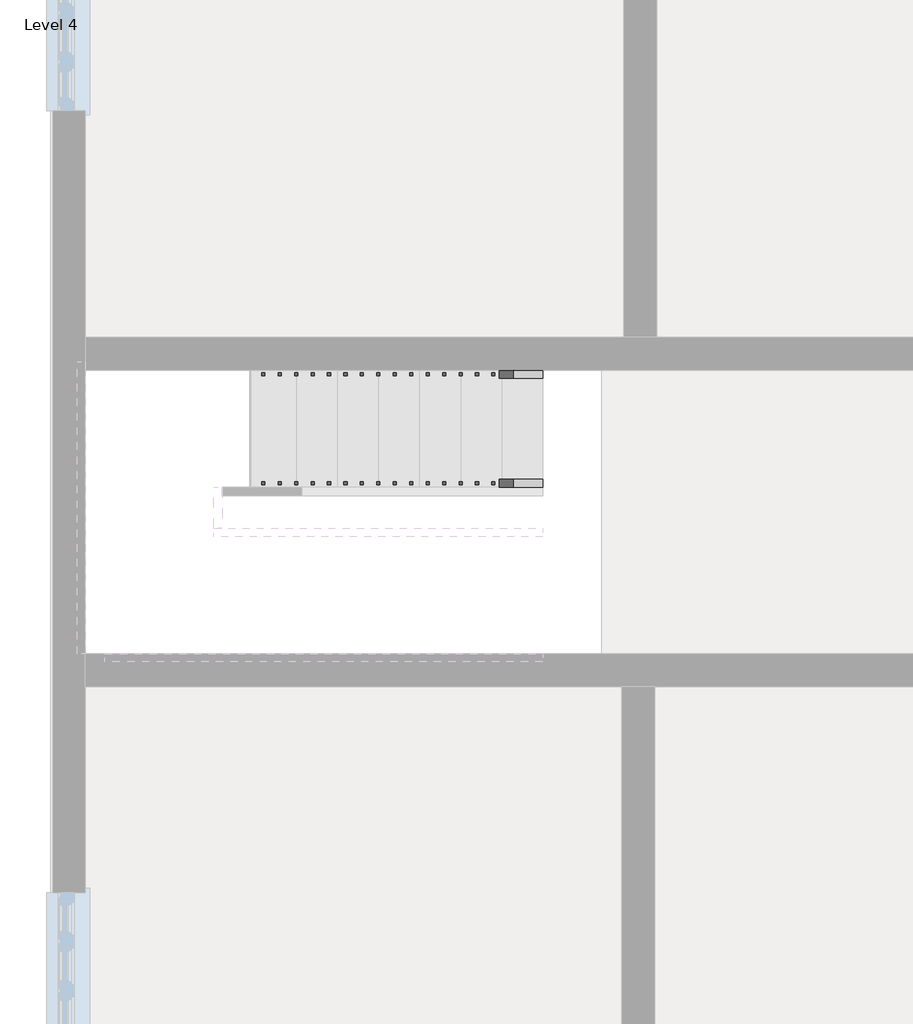
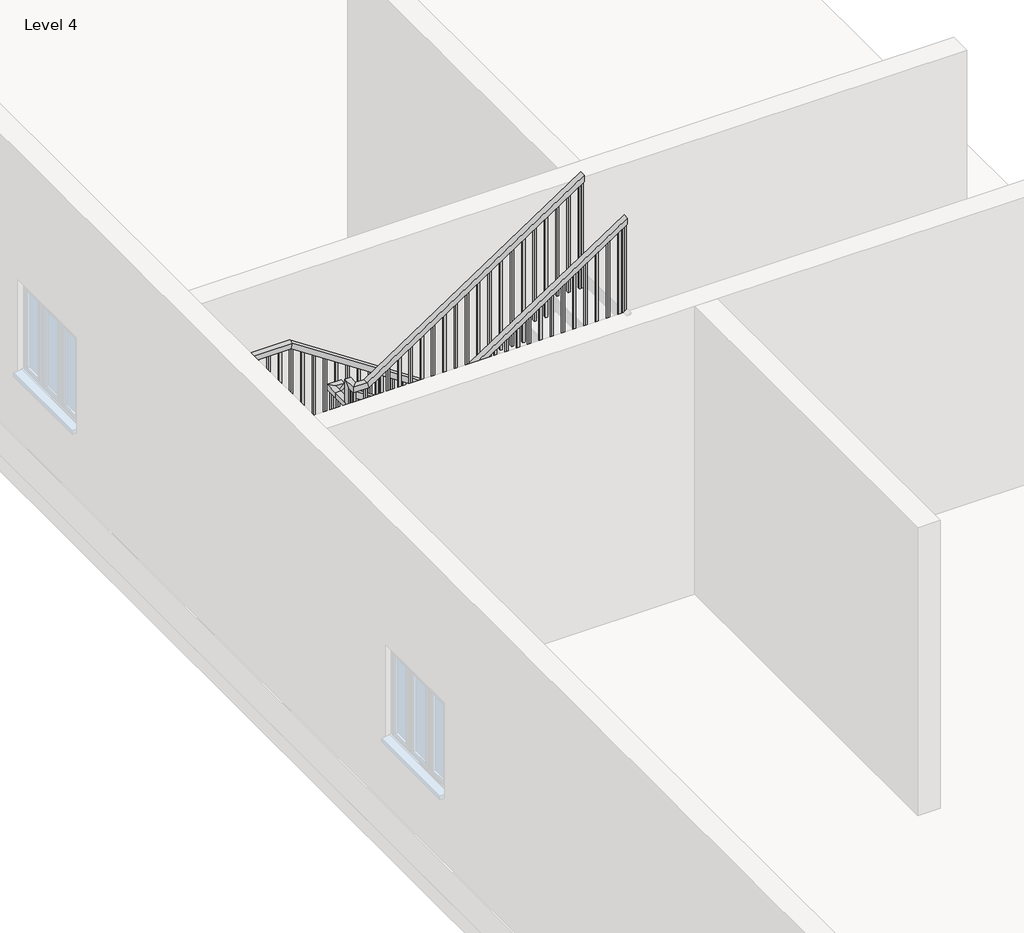
# One storey, part 2 of 3: 2 railings.
"""IFC4 building model written with IfcOpenShell, lengths in millimetres."""

from ifc_helpers import new_model, si_unit, frame, origin, place, context, project, spatial, polyline, outline, extrude, faceted_brep, element, save

model = new_model("IFC4")

# Units and contexts
model_context = context("Model", 3, world=origin())
ifc_project = project(units=[si_unit("LENGTHUNIT", "METRE", prefix="MILLI")], contexts=[model_context])

# Site, building, storey
site = spatial("IfcSite", under=ifc_project)
building = spatial("IfcBuilding", under=site)
storey = spatial("IfcBuildingStorey", under=building, Name="Level 4", Elevation=9144.0)

# Railings
placement = place(None, origin())
element("IfcRailing", 1, ObjectType="Handrail - Rectangular", at=placement, inside=storey, context=model_context, shape_type="SolidModel", body=[
    faceted_brep([(-2118.1728655, 1141.7797121, 10226.3222222), (-2118.1728655, 1141.7797121, 10165.4243166), (-2118.1728655, 1192.5797121, 10165.4243166), (-2118.1728655, 1192.5797121, 10226.3222222), (-4150.1728655, 1141.7797121, 11569.7), (-4165.4470084, 1141.7797121, 11518.9), (-4165.4470084, 1192.5797121, 11518.9), (-4150.1728655, 1192.5797121, 11569.7), (-4893.1394105, 1141.7797121, 11569.7), (-4893.1394105, 1141.7797121, 11518.9), (-4943.9394105, 1192.5797121, 11518.9), (-4943.9394105, 1192.5797121, 11569.7), (-4893.1394105, -509.2202879, 11569.7), (-4893.1394105, -509.2202879, 11518.9), (-4943.9394105, -560.0202879, 11518.9), (-4943.9394105, -560.0202879, 11569.7), (-4404.1728655, -509.2202879, 11569.7), (-4388.8987225, -509.2202879, 11518.9), (-4388.8987225, -560.0202879, 11518.9), (-4404.1728655, -560.0202879, 11569.7), (-2118.1728655, -509.2202879, 13081.0), (-2118.1728655, -560.0202879, 13081.0), (-2118.1728655, -560.0202879, 13020.1020944), (-2118.1728655, -509.2202879, 13020.1020944)], [[[0, 1, 2, 3]], [[1, 0, 4, 5]], [[2, 1, 5, 6]], [[3, 2, 6, 7]], [[0, 3, 7, 4]], [[5, 4, 8, 9]], [[6, 5, 9, 10]], [[7, 6, 10, 11]], [[4, 7, 11, 8]], [[9, 8, 12, 13]], [[10, 9, 13, 14]], [[11, 10, 14, 15]], [[8, 11, 15, 12]], [[13, 12, 16, 17]], [[14, 13, 17, 18]], [[15, 14, 18, 19]], [[12, 15, 19, 16]], [[20, 21, 22, 23]], [[17, 16, 20, 23]], [[18, 17, 23, 22]], [[19, 18, 22, 21]], [[16, 19, 21, 20]]]),
    extrude(outline(polyline([(12988.6057396, -2165.8144105), (12976.0115729, -2184.8644105), (11998.6777778, -2184.8644105), (11998.6777778, -2165.8144105), (12988.6057396, -2165.8144105)])), frame((0.0, -544.1452879, 0.0), z_axis=(0.0, 1.0, 0.0), x_axis=(0.0, 0.0, 1.0)), (0.0, 0.0, 1.0), 19.05),
    extrude(outline(polyline([(12921.4368507, -2267.4144105), (12908.842684, -2286.4644105), (11998.6777778, -2286.4644105), (11998.6777778, -2267.4144105), (12921.4368507, -2267.4144105)])), frame((0.0, -544.1452879, 0.0), z_axis=(0.0, 1.0, 0.0), x_axis=(0.0, 0.0, 1.0)), (0.0, 0.0, 1.0), 19.05),
    extrude(outline(polyline([(12854.2679618, -2369.0144105), (12841.6737951, -2388.0644105), (11830.7555556, -2388.0644105), (11830.7555556, -2369.0144105), (12854.2679618, -2369.0144105)])), frame((0.0, -544.1452879, 0.0), z_axis=(0.0, 1.0, 0.0), x_axis=(0.0, 0.0, 1.0)), (0.0, 0.0, 1.0), 19.05),
    extrude(outline(polyline([(12787.0990729, -2470.6144105), (12774.5049062, -2489.6644105), (11830.7555556, -2489.6644105), (11830.7555556, -2470.6144105), (12787.0990729, -2470.6144105)])), frame((0.0, -544.1452879, 0.0), z_axis=(0.0, 1.0, 0.0), x_axis=(0.0, 0.0, 1.0)), (0.0, 0.0, 1.0), 19.05),
    extrude(outline(polyline([(12719.930184, -2572.2144105), (12707.3360174, -2591.2644105), (11830.7555556, -2591.2644105), (11830.7555556, -2572.2144105), (12719.930184, -2572.2144105)])), frame((0.0, -544.1452879, 0.0), z_axis=(0.0, 1.0, 0.0), x_axis=(0.0, 0.0, 1.0)), (0.0, 0.0, 1.0), 19.05),
    extrude(outline(polyline([(12652.7612951, -2673.8144105), (12640.1671285, -2692.8644105), (11662.8333333, -2692.8644105), (11662.8333333, -2673.8144105), (12652.7612951, -2673.8144105)])), frame((0.0, -544.1452879, 0.0), z_axis=(0.0, 1.0, 0.0), x_axis=(0.0, 0.0, 1.0)), (0.0, 0.0, 1.0), 19.05),
    extrude(outline(polyline([(12585.5924062, -2775.4144105), (12572.9982396, -2794.4644105), (11662.8333333, -2794.4644105), (11662.8333333, -2775.4144105), (12585.5924062, -2775.4144105)])), frame((0.0, -544.1452879, 0.0), z_axis=(0.0, 1.0, 0.0), x_axis=(0.0, 0.0, 1.0)), (0.0, 0.0, 1.0), 19.05),
    extrude(outline(polyline([(12518.4235174, -2877.0144105), (12505.8293507, -2896.0644105), (11494.9111111, -2896.0644105), (11494.9111111, -2877.0144105), (12518.4235174, -2877.0144105)])), frame((0.0, -544.1452879, 0.0), z_axis=(0.0, 1.0, 0.0), x_axis=(0.0, 0.0, 1.0)), (0.0, 0.0, 1.0), 19.05),
    extrude(outline(polyline([(12451.2546285, -2978.6144105), (12438.6604618, -2997.6644105), (11494.9111111, -2997.6644105), (11494.9111111, -2978.6144105), (12451.2546285, -2978.6144105)])), frame((0.0, -544.1452879, 0.0), z_axis=(0.0, 1.0, 0.0), x_axis=(0.0, 0.0, 1.0)), (0.0, 0.0, 1.0), 19.05),
    extrude(outline(polyline([(12384.0857396, -3080.2144105), (12371.4915729, -3099.2644105), (11494.9111111, -3099.2644105), (11494.9111111, -3080.2144105), (12384.0857396, -3080.2144105)])), frame((0.0, -544.1452879, 0.0), z_axis=(0.0, 1.0, 0.0), x_axis=(0.0, 0.0, 1.0)), (0.0, 0.0, 1.0), 19.05),
    extrude(outline(polyline([(12316.9168507, -3181.8144105), (12304.322684, -3200.8644105), (11326.9888889, -3200.8644105), (11326.9888889, -3181.8144105), (12316.9168507, -3181.8144105)])), frame((0.0, -544.1452879, 0.0), z_axis=(0.0, 1.0, 0.0), x_axis=(0.0, 0.0, 1.0)), (0.0, 0.0, 1.0), 19.05),
    extrude(outline(polyline([(12249.7479618, -3283.4144105), (12237.1537951, -3302.4644105), (11326.9888889, -3302.4644105), (11326.9888889, -3283.4144105), (12249.7479618, -3283.4144105)])), frame((0.0, -544.1452879, 0.0), z_axis=(0.0, 1.0, 0.0), x_axis=(0.0, 0.0, 1.0)), (0.0, 0.0, 1.0), 19.05),
    extrude(outline(polyline([(12182.5790729, -3385.0144105), (12169.9849062, -3404.0644105), (11159.0666667, -3404.0644105), (11159.0666667, -3385.0144105), (12182.5790729, -3385.0144105)])), frame((0.0, -544.1452879, 0.0), z_axis=(0.0, 1.0, 0.0), x_axis=(0.0, 0.0, 1.0)), (0.0, 0.0, 1.0), 19.05),
    extrude(outline(polyline([(12115.410184, -3486.6144105), (12102.8160174, -3505.6644105), (11159.0666667, -3505.6644105), (11159.0666667, -3486.6144105), (12115.410184, -3486.6144105)])), frame((0.0, -544.1452879, 0.0), z_axis=(0.0, 1.0, 0.0), x_axis=(0.0, 0.0, 1.0)), (0.0, 0.0, 1.0), 19.05),
    extrude(outline(polyline([(12048.2412951, -3588.2144105), (12035.6471285, -3607.2644105), (11159.0666667, -3607.2644105), (11159.0666667, -3588.2144105), (12048.2412951, -3588.2144105)])), frame((0.0, -544.1452879, 0.0), z_axis=(0.0, 1.0, 0.0), x_axis=(0.0, 0.0, 1.0)), (0.0, 0.0, 1.0), 19.05),
    extrude(outline(polyline([(11981.0724062, -3689.8144105), (11968.4782396, -3708.8644105), (10991.1444444, -3708.8644105), (10991.1444444, -3689.8144105), (11981.0724062, -3689.8144105)])), frame((0.0, -544.1452879, 0.0), z_axis=(0.0, 1.0, 0.0), x_axis=(0.0, 0.0, 1.0)), (0.0, 0.0, 1.0), 19.05),
    extrude(outline(polyline([(11913.9035174, -3791.4144105), (11901.3093507, -3810.4644105), (10991.1444444, -3810.4644105), (10991.1444444, -3791.4144105), (11913.9035174, -3791.4144105)])), frame((0.0, -544.1452879, 0.0), z_axis=(0.0, 1.0, 0.0), x_axis=(0.0, 0.0, 1.0)), (0.0, 0.0, 1.0), 19.05),
    extrude(outline(polyline([(11846.7346285, -3893.0144105), (11834.1404618, -3912.0644105), (10823.2222222, -3912.0644105), (10823.2222222, -3893.0144105), (11846.7346285, -3893.0144105)])), frame((0.0, -544.1452879, 0.0), z_axis=(0.0, 1.0, 0.0), x_axis=(0.0, 0.0, 1.0)), (0.0, 0.0, 1.0), 19.05),
    extrude(outline(polyline([(11779.5657396, -3994.6144105), (11766.9715729, -4013.6644105), (10823.2222222, -4013.6644105), (10823.2222222, -3994.6144105), (11779.5657396, -3994.6144105)])), frame((0.0, -544.1452879, 0.0), z_axis=(0.0, 1.0, 0.0), x_axis=(0.0, 0.0, 1.0)), (0.0, 0.0, 1.0), 19.05),
    extrude(outline(polyline([(11712.3968507, -4096.2144105), (11699.802684, -4115.2644105), (10823.2222222, -4115.2644105), (10823.2222222, -4096.2144105), (11712.3968507, -4096.2144105)])), frame((0.0, -544.1452879, 0.0), z_axis=(0.0, 1.0, 0.0), x_axis=(0.0, 0.0, 1.0)), (0.0, 0.0, 1.0), 19.05),
    extrude(outline(polyline([(11645.2279618, -4197.8144105), (11632.6337951, -4216.8644105), (10655.3, -4216.8644105), (10655.3, -4197.8144105), (11645.2279618, -4197.8144105)])), frame((0.0, -544.1452879, 0.0), z_axis=(0.0, 1.0, 0.0), x_axis=(0.0, 0.0, 1.0)), (0.0, 0.0, 1.0), 19.05),
    extrude(outline(polyline([(11578.0590729, -4299.4144105), (11565.4649062, -4318.4644105), (10655.3, -4318.4644105), (10655.3, -4299.4144105), (11578.0590729, -4299.4144105)])), frame((0.0, -544.1452879, 0.0), z_axis=(0.0, 1.0, 0.0), x_axis=(0.0, 0.0, 1.0)), (0.0, 0.0, 1.0), 19.05),
    extrude(outline(polyline([(-4420.0644105, -544.1452879), (-4420.0644105, -525.0952879), (-4401.0144105, -525.0952879), (-4401.0144105, -544.1452879), (-4420.0644105, -544.1452879)])), frame((0.0, 0.0, 10655.3), z_axis=(0.0, 0.0, 1.0), x_axis=(1.0, 0.0, 0.0)), (0.0, 0.0, 1.0), 863.6),
    extrude(outline(polyline([(-4521.6644105, -544.1452879), (-4521.6644105, -525.0952879), (-4502.6144105, -525.0952879), (-4502.6144105, -544.1452879), (-4521.6644105, -544.1452879)])), frame((0.0, 0.0, 10655.3), z_axis=(0.0, 0.0, 1.0), x_axis=(1.0, 0.0, 0.0)), (0.0, 0.0, 1.0), 863.6),
    extrude(outline(polyline([(-4623.2644105, -544.1452879), (-4623.2644105, -525.0952879), (-4604.2144105, -525.0952879), (-4604.2144105, -544.1452879), (-4623.2644105, -544.1452879)])), frame((0.0, 0.0, 10655.3), z_axis=(0.0, 0.0, 1.0), x_axis=(1.0, 0.0, 0.0)), (0.0, 0.0, 1.0), 863.6),
    extrude(outline(polyline([(-4724.8644105, -544.1452879), (-4724.8644105, -525.0952879), (-4705.8144105, -525.0952879), (-4705.8144105, -544.1452879), (-4724.8644105, -544.1452879)])), frame((0.0, 0.0, 10655.3), z_axis=(0.0, 0.0, 1.0), x_axis=(1.0, 0.0, 0.0)), (0.0, 0.0, 1.0), 863.6),
    extrude(outline(polyline([(-4826.4644105, -544.1452879), (-4826.4644105, -525.0952879), (-4807.4144105, -525.0952879), (-4807.4144105, -544.1452879), (-4826.4644105, -544.1452879)])), frame((0.0, 0.0, 10655.3), z_axis=(0.0, 0.0, 1.0), x_axis=(1.0, 0.0, 0.0)), (0.0, 0.0, 1.0), 863.6),
    extrude(outline(polyline([(-4928.0644105, -448.8952879), (-4909.0144105, -448.8952879), (-4909.0144105, -467.9452879), (-4928.0644105, -467.9452879), (-4928.0644105, -448.8952879)])), frame((0.0, 0.0, 10655.3), z_axis=(0.0, 0.0, 1.0), x_axis=(1.0, 0.0, 0.0)), (0.0, 0.0, 1.0), 863.6),
    extrude(outline(polyline([(-4928.0644105, -347.2952879), (-4909.0144105, -347.2952879), (-4909.0144105, -366.3452879), (-4928.0644105, -366.3452879), (-4928.0644105, -347.2952879)])), frame((0.0, 0.0, 10655.3), z_axis=(0.0, 0.0, 1.0), x_axis=(1.0, 0.0, 0.0)), (0.0, 0.0, 1.0), 863.6),
    extrude(outline(polyline([(-4928.0644105, -245.6952879), (-4909.0144105, -245.6952879), (-4909.0144105, -264.7452879), (-4928.0644105, -264.7452879), (-4928.0644105, -245.6952879)])), frame((0.0, 0.0, 10655.3), z_axis=(0.0, 0.0, 1.0), x_axis=(1.0, 0.0, 0.0)), (0.0, 0.0, 1.0), 863.6),
    extrude(outline(polyline([(-4928.0644105, -144.0952879), (-4909.0144105, -144.0952879), (-4909.0144105, -163.1452879), (-4928.0644105, -163.1452879), (-4928.0644105, -144.0952879)])), frame((0.0, 0.0, 10655.3), z_axis=(0.0, 0.0, 1.0), x_axis=(1.0, 0.0, 0.0)), (0.0, 0.0, 1.0), 863.6),
    extrude(outline(polyline([(-4928.0644105, -42.4952879), (-4909.0144105, -42.4952879), (-4909.0144105, -61.5452879), (-4928.0644105, -61.5452879), (-4928.0644105, -42.4952879)])), frame((0.0, 0.0, 10655.3), z_axis=(0.0, 0.0, 1.0), x_axis=(1.0, 0.0, 0.0)), (0.0, 0.0, 1.0), 863.6),
    extrude(outline(polyline([(-4928.0644105, 59.1047121), (-4909.0144105, 59.1047121), (-4909.0144105, 40.0547121), (-4928.0644105, 40.0547121), (-4928.0644105, 59.1047121)])), frame((0.0, 0.0, 10655.3), z_axis=(0.0, 0.0, 1.0), x_axis=(1.0, 0.0, 0.0)), (0.0, 0.0, 1.0), 863.6),
    extrude(outline(polyline([(-4928.0644105, 160.7047121), (-4909.0144105, 160.7047121), (-4909.0144105, 141.6547121), (-4928.0644105, 141.6547121), (-4928.0644105, 160.7047121)])), frame((0.0, 0.0, 10655.3), z_axis=(0.0, 0.0, 1.0), x_axis=(1.0, 0.0, 0.0)), (0.0, 0.0, 1.0), 863.6),
    extrude(outline(polyline([(-4928.0644105, 262.3047121), (-4909.0144105, 262.3047121), (-4909.0144105, 243.2547121), (-4928.0644105, 243.2547121), (-4928.0644105, 262.3047121)])), frame((0.0, 0.0, 10655.3), z_axis=(0.0, 0.0, 1.0), x_axis=(1.0, 0.0, 0.0)), (0.0, 0.0, 1.0), 863.6),
    extrude(outline(polyline([(-4928.0644105, 363.9047121), (-4909.0144105, 363.9047121), (-4909.0144105, 344.8547121), (-4928.0644105, 344.8547121), (-4928.0644105, 363.9047121)])), frame((0.0, 0.0, 10655.3), z_axis=(0.0, 0.0, 1.0), x_axis=(1.0, 0.0, 0.0)), (0.0, 0.0, 1.0), 863.6),
    extrude(outline(polyline([(-4928.0644105, 465.5047121), (-4909.0144105, 465.5047121), (-4909.0144105, 446.4547121), (-4928.0644105, 446.4547121), (-4928.0644105, 465.5047121)])), frame((0.0, 0.0, 10655.3), z_axis=(0.0, 0.0, 1.0), x_axis=(1.0, 0.0, 0.0)), (0.0, 0.0, 1.0), 863.6),
    extrude(outline(polyline([(-4928.0644105, 567.1047121), (-4909.0144105, 567.1047121), (-4909.0144105, 548.0547121), (-4928.0644105, 548.0547121), (-4928.0644105, 567.1047121)])), frame((0.0, 0.0, 10655.3), z_axis=(0.0, 0.0, 1.0), x_axis=(1.0, 0.0, 0.0)), (0.0, 0.0, 1.0), 863.6),
    extrude(outline(polyline([(-4928.0644105, 668.7047121), (-4909.0144105, 668.7047121), (-4909.0144105, 649.6547121), (-4928.0644105, 649.6547121), (-4928.0644105, 668.7047121)])), frame((0.0, 0.0, 10655.3), z_axis=(0.0, 0.0, 1.0), x_axis=(1.0, 0.0, 0.0)), (0.0, 0.0, 1.0), 863.6),
    extrude(outline(polyline([(-4928.0644105, 770.3047121), (-4909.0144105, 770.3047121), (-4909.0144105, 751.2547121), (-4928.0644105, 751.2547121), (-4928.0644105, 770.3047121)])), frame((0.0, 0.0, 10655.3), z_axis=(0.0, 0.0, 1.0), x_axis=(1.0, 0.0, 0.0)), (0.0, 0.0, 1.0), 863.6),
    extrude(outline(polyline([(-4928.0644105, 871.9047121), (-4909.0144105, 871.9047121), (-4909.0144105, 852.8547121), (-4928.0644105, 852.8547121), (-4928.0644105, 871.9047121)])), frame((0.0, 0.0, 10655.3), z_axis=(0.0, 0.0, 1.0), x_axis=(1.0, 0.0, 0.0)), (0.0, 0.0, 1.0), 863.6),
    extrude(outline(polyline([(-4928.0644105, 973.5047121), (-4909.0144105, 973.5047121), (-4909.0144105, 954.4547121), (-4928.0644105, 954.4547121), (-4928.0644105, 973.5047121)])), frame((0.0, 0.0, 10655.3), z_axis=(0.0, 0.0, 1.0), x_axis=(1.0, 0.0, 0.0)), (0.0, 0.0, 1.0), 863.6),
    extrude(outline(polyline([(-4928.0644105, 1075.1047121), (-4909.0144105, 1075.1047121), (-4909.0144105, 1056.0547121), (-4928.0644105, 1056.0547121), (-4928.0644105, 1075.1047121)])), frame((0.0, 0.0, 10655.3), z_axis=(0.0, 0.0, 1.0), x_axis=(1.0, 0.0, 0.0)), (0.0, 0.0, 1.0), 863.6),
    extrude(outline(polyline([(-4851.8478655, 1176.7047121), (-4851.8478655, 1157.6547121), (-4870.8978655, 1157.6547121), (-4870.8978655, 1176.7047121), (-4851.8478655, 1176.7047121)])), frame((0.0, 0.0, 10655.3), z_axis=(0.0, 0.0, 1.0), x_axis=(1.0, 0.0, 0.0)), (0.0, 0.0, 1.0), 863.6),
    extrude(outline(polyline([(-4750.2478655, 1176.7047121), (-4750.2478655, 1157.6547121), (-4769.2978655, 1157.6547121), (-4769.2978655, 1176.7047121), (-4750.2478655, 1176.7047121)])), frame((0.0, 0.0, 10655.3), z_axis=(0.0, 0.0, 1.0), x_axis=(1.0, 0.0, 0.0)), (0.0, 0.0, 1.0), 863.6),
    extrude(outline(polyline([(-4648.6478655, 1176.7047121), (-4648.6478655, 1157.6547121), (-4667.6978655, 1157.6547121), (-4667.6978655, 1176.7047121), (-4648.6478655, 1176.7047121)])), frame((0.0, 0.0, 10655.3), z_axis=(0.0, 0.0, 1.0), x_axis=(1.0, 0.0, 0.0)), (0.0, 0.0, 1.0), 863.6),
    extrude(outline(polyline([(-4547.0478655, 1176.7047121), (-4547.0478655, 1157.6547121), (-4566.0978655, 1157.6547121), (-4566.0978655, 1176.7047121), (-4547.0478655, 1176.7047121)])), frame((0.0, 0.0, 10655.3), z_axis=(0.0, 0.0, 1.0), x_axis=(1.0, 0.0, 0.0)), (0.0, 0.0, 1.0), 863.6),
    extrude(outline(polyline([(-4445.4478655, 1176.7047121), (-4445.4478655, 1157.6547121), (-4464.4978655, 1157.6547121), (-4464.4978655, 1176.7047121), (-4445.4478655, 1176.7047121)])), frame((0.0, 0.0, 10655.3), z_axis=(0.0, 0.0, 1.0), x_axis=(1.0, 0.0, 0.0)), (0.0, 0.0, 1.0), 863.6),
    extrude(outline(polyline([(-4343.8478655, 1176.7047121), (-4343.8478655, 1157.6547121), (-4362.8978655, 1157.6547121), (-4362.8978655, 1176.7047121), (-4343.8478655, 1176.7047121)])), frame((0.0, 0.0, 10655.3), z_axis=(0.0, 0.0, 1.0), x_axis=(1.0, 0.0, 0.0)), (0.0, 0.0, 1.0), 863.6),
    extrude(outline(polyline([(-4242.2478655, 1176.7047121), (-4242.2478655, 1157.6547121), (-4261.2978655, 1157.6547121), (-4261.2978655, 1176.7047121), (-4242.2478655, 1176.7047121)])), frame((0.0, 0.0, 10655.3), z_axis=(0.0, 0.0, 1.0), x_axis=(1.0, 0.0, 0.0)), (0.0, 0.0, 1.0), 863.6),
    extrude(outline(polyline([(11502.505011, -4140.6478655), (11515.0991777, -4159.6978655), (10655.3, -4159.6978655), (10655.3, -4140.6478655), (11502.505011, -4140.6478655)])), frame((0.0, 1157.6547121, 0.0), z_axis=(0.0, 1.0, 0.0), x_axis=(0.0, 0.0, 1.0)), (0.0, 0.0, 1.0), 19.05),
    extrude(outline(polyline([(11435.3361222, -4039.0478655), (11447.9302888, -4058.0978655), (10487.3777778, -4058.0978655), (10487.3777778, -4039.0478655), (11435.3361222, -4039.0478655)])), frame((0.0, 1157.6547121, 0.0), z_axis=(0.0, 1.0, 0.0), x_axis=(0.0, 0.0, 1.0)), (0.0, 0.0, 1.0), 19.05),
    extrude(outline(polyline([(11368.1672333, -3937.4478655), (11380.7613999, -3956.4978655), (10487.3777778, -3956.4978655), (10487.3777778, -3937.4478655), (11368.1672333, -3937.4478655)])), frame((0.0, 1157.6547121, 0.0), z_axis=(0.0, 1.0, 0.0), x_axis=(0.0, 0.0, 1.0)), (0.0, 0.0, 1.0), 19.05),
    extrude(outline(polyline([(11300.9983444, -3835.8478655), (11313.592511, -3854.8978655), (10319.4555556, -3854.8978655), (10319.4555556, -3835.8478655), (11300.9983444, -3835.8478655)])), frame((0.0, 1157.6547121, 0.0), z_axis=(0.0, 1.0, 0.0), x_axis=(0.0, 0.0, 1.0)), (0.0, 0.0, 1.0), 19.05),
    extrude(outline(polyline([(11233.8294555, -3734.2478655), (11246.4236222, -3753.2978655), (10319.4555556, -3753.2978655), (10319.4555556, -3734.2478655), (11233.8294555, -3734.2478655)])), frame((0.0, 1157.6547121, 0.0), z_axis=(0.0, 1.0, 0.0), x_axis=(0.0, 0.0, 1.0)), (0.0, 0.0, 1.0), 19.05),
    extrude(outline(polyline([(11166.6605666, -3632.6478655), (11179.2547333, -3651.6978655), (10319.4555556, -3651.6978655), (10319.4555556, -3632.6478655), (11166.6605666, -3632.6478655)])), frame((0.0, 1157.6547121, 0.0), z_axis=(0.0, 1.0, 0.0), x_axis=(0.0, 0.0, 1.0)), (0.0, 0.0, 1.0), 19.05),
    extrude(outline(polyline([(11099.4916777, -3531.0478655), (11112.0858444, -3550.0978655), (10151.5333333, -3550.0978655), (10151.5333333, -3531.0478655), (11099.4916777, -3531.0478655)])), frame((0.0, 1157.6547121, 0.0), z_axis=(0.0, 1.0, 0.0), x_axis=(0.0, 0.0, 1.0)), (0.0, 0.0, 1.0), 19.05),
    extrude(outline(polyline([(11032.3227888, -3429.4478655), (11044.9169555, -3448.4978655), (10151.5333333, -3448.4978655), (10151.5333333, -3429.4478655), (11032.3227888, -3429.4478655)])), frame((0.0, 1157.6547121, 0.0), z_axis=(0.0, 1.0, 0.0), x_axis=(0.0, 0.0, 1.0)), (0.0, 0.0, 1.0), 19.05),
    extrude(outline(polyline([(10965.1538999, -3327.8478655), (10977.7480666, -3346.8978655), (9983.6111111, -3346.8978655), (9983.6111111, -3327.8478655), (10965.1538999, -3327.8478655)])), frame((0.0, 1157.6547121, 0.0), z_axis=(0.0, 1.0, 0.0), x_axis=(0.0, 0.0, 1.0)), (0.0, 0.0, 1.0), 19.05),
    extrude(outline(polyline([(10897.985011, -3226.2478655), (10910.5791777, -3245.2978655), (9983.6111111, -3245.2978655), (9983.6111111, -3226.2478655), (10897.985011, -3226.2478655)])), frame((0.0, 1157.6547121, 0.0), z_axis=(0.0, 1.0, 0.0), x_axis=(0.0, 0.0, 1.0)), (0.0, 0.0, 1.0), 19.05),
    extrude(outline(polyline([(10830.8161222, -3124.6478655), (10843.4102888, -3143.6978655), (9983.6111111, -3143.6978655), (9983.6111111, -3124.6478655), (10830.8161222, -3124.6478655)])), frame((0.0, 1157.6547121, 0.0), z_axis=(0.0, 1.0, 0.0), x_axis=(0.0, 0.0, 1.0)), (0.0, 0.0, 1.0), 19.05),
    extrude(outline(polyline([(10763.6472333, -3023.0478655), (10776.2413999, -3042.0978655), (9815.6888889, -3042.0978655), (9815.6888889, -3023.0478655), (10763.6472333, -3023.0478655)])), frame((0.0, 1157.6547121, 0.0), z_axis=(0.0, 1.0, 0.0), x_axis=(0.0, 0.0, 1.0)), (0.0, 0.0, 1.0), 19.05),
    extrude(outline(polyline([(10696.4783444, -2921.4478655), (10709.072511, -2940.4978655), (9815.6888889, -2940.4978655), (9815.6888889, -2921.4478655), (10696.4783444, -2921.4478655)])), frame((0.0, 1157.6547121, 0.0), z_axis=(0.0, 1.0, 0.0), x_axis=(0.0, 0.0, 1.0)), (0.0, 0.0, 1.0), 19.05),
    extrude(outline(polyline([(10629.3094555, -2819.8478655), (10641.9036222, -2838.8978655), (9647.7666667, -2838.8978655), (9647.7666667, -2819.8478655), (10629.3094555, -2819.8478655)])), frame((0.0, 1157.6547121, 0.0), z_axis=(0.0, 1.0, 0.0), x_axis=(0.0, 0.0, 1.0)), (0.0, 0.0, 1.0), 19.05),
    extrude(outline(polyline([(10562.1405666, -2718.2478655), (10574.7347333, -2737.2978655), (9647.7666667, -2737.2978655), (9647.7666667, -2718.2478655), (10562.1405666, -2718.2478655)])), frame((0.0, 1157.6547121, 0.0), z_axis=(0.0, 1.0, 0.0), x_axis=(0.0, 0.0, 1.0)), (0.0, 0.0, 1.0), 19.05),
    extrude(outline(polyline([(10494.9716777, -2616.6478655), (10507.5658444, -2635.6978655), (9647.7666667, -2635.6978655), (9647.7666667, -2616.6478655), (10494.9716777, -2616.6478655)])), frame((0.0, 1157.6547121, 0.0), z_axis=(0.0, 1.0, 0.0), x_axis=(0.0, 0.0, 1.0)), (0.0, 0.0, 1.0), 19.05),
    extrude(outline(polyline([(10427.8027888, -2515.0478655), (10440.3969555, -2534.0978655), (9479.8444444, -2534.0978655), (9479.8444444, -2515.0478655), (10427.8027888, -2515.0478655)])), frame((0.0, 1157.6547121, 0.0), z_axis=(0.0, 1.0, 0.0), x_axis=(0.0, 0.0, 1.0)), (0.0, 0.0, 1.0), 19.05),
    extrude(outline(polyline([(10360.6338999, -2413.4478655), (10373.2280666, -2432.4978655), (9479.8444444, -2432.4978655), (9479.8444444, -2413.4478655), (10360.6338999, -2413.4478655)])), frame((0.0, 1157.6547121, 0.0), z_axis=(0.0, 1.0, 0.0), x_axis=(0.0, 0.0, 1.0)), (0.0, 0.0, 1.0), 19.05),
    extrude(outline(polyline([(10293.465011, -2311.8478655), (10306.0591777, -2330.8978655), (9311.9222222, -2330.8978655), (9311.9222222, -2311.8478655), (10293.465011, -2311.8478655)])), frame((0.0, 1157.6547121, 0.0), z_axis=(0.0, 1.0, 0.0), x_axis=(0.0, 0.0, 1.0)), (0.0, 0.0, 1.0), 19.05),
    extrude(outline(polyline([(10226.2961222, -2210.2478655), (10238.8902888, -2229.2978655), (9311.9222222, -2229.2978655), (9311.9222222, -2210.2478655), (10226.2961222, -2210.2478655)])), frame((0.0, 1157.6547121, 0.0), z_axis=(0.0, 1.0, 0.0), x_axis=(0.0, 0.0, 1.0)), (0.0, 0.0, 1.0), 19.05),
    extrude(outline(polyline([(-4928.0644105, -525.0952879), (-4909.0144105, -525.0952879), (-4909.0144105, -544.1452879), (-4928.0644105, -544.1452879), (-4928.0644105, -525.0952879)])), frame((0.0, 0.0, 10655.3), z_axis=(0.0, 0.0, 1.0), x_axis=(1.0, 0.0, 0.0)), (0.0, 0.0, 1.0), 863.6),
    extrude(outline(polyline([(-4909.0144105, 1176.7047121), (-4909.0144105, 1157.6547121), (-4928.0644105, 1157.6547121), (-4928.0644105, 1176.7047121), (-4909.0144105, 1176.7047121)])), frame((0.0, 0.0, 10655.3), z_axis=(0.0, 0.0, 1.0), x_axis=(1.0, 0.0, 0.0)), (0.0, 0.0, 1.0), 863.6),
    extrude(outline(polyline([(13020.1020944, -2118.1728655), (13007.5079277, -2137.2228655), (11998.6777778, -2137.2228655), (11998.6777778, -2118.1728655), (13020.1020944, -2118.1728655)])), frame((0.0, -544.1452879, 0.0), z_axis=(0.0, 1.0, 0.0), x_axis=(0.0, 0.0, 1.0)), (0.0, 0.0, 1.0), 19.05),
    extrude(outline(polyline([(10165.4243166, -2118.1728655), (10178.0184833, -2137.2228655), (9311.9222222, -2137.2228655), (9311.9222222, -2118.1728655), (10165.4243166, -2118.1728655)])), frame((0.0, 1157.6547121, 0.0), z_axis=(0.0, 1.0, 0.0), x_axis=(0.0, 0.0, 1.0)), (0.0, 0.0, 1.0), 19.05),
])
element("IfcRailing", 2, ObjectType="Handrail - Rectangular", at=placement, inside=storey, context=model_context, shape_type="SolidModel", body=[
    faceted_brep([(-2118.1728655, 468.6797121, 10226.3222222), (-2118.1728655, 468.6797121, 10165.4243166), (-2118.1728655, 519.4797121, 10165.4243166), (-2118.1728655, 519.4797121, 10226.3222222), (-4073.9728655, 468.6797121, 11519.3233333), (-4124.7728655, 468.6797121, 11492.0098722), (-4124.7728655, 519.4797121, 11492.0098722), (-4073.9728655, 519.4797121, 11519.3233333), (-4073.9728655, 468.6797121, 11569.7), (-4124.7728655, 468.6797121, 11518.9), (-4124.7728655, 519.4797121, 11518.9), (-4073.9728655, 519.4797121, 11569.7), (-4150.1728655, 468.6797121, 11569.7), (-4150.1728655, 468.6797121, 11518.9), (-4200.9728655, 519.4797121, 11518.9), (-4200.9728655, 519.4797121, 11569.7), (-4150.1728655, 392.4797121, 11569.7), (-4150.1728655, 392.4797121, 11518.9), (-4200.9728655, 392.4797121, 11518.9), (-4200.9728655, 392.4797121, 11569.7), (-4150.1728655, 240.0797121, 11569.7), (-4150.1728655, 189.2797121, 11518.9), (-4200.9728655, 189.2797121, 11518.9), (-4200.9728655, 240.0797121, 11569.7), (-4150.1728655, 240.0797121, 11787.9988889), (-4150.1728655, 189.2797121, 11737.1988889), (-4200.9728655, 189.2797121, 11737.1988889), (-4200.9728655, 240.0797121, 11787.9988889), (-4150.1728655, 163.8797121, 11787.9988889), (-4150.1728655, 163.8797121, 11737.1988889), (-4200.9728655, 113.0797121, 11737.1988889), (-4200.9728655, 113.0797121, 11787.9988889), (-4073.9728655, 163.8797121, 11787.9988889), (-4058.6987225, 163.8797121, 11737.1988889), (-4058.6987225, 113.0797121, 11737.1988889), (-4073.9728655, 113.0797121, 11787.9988889), (-2118.1728655, 163.8797121, 13081.0), (-2118.1728655, 113.0797121, 13081.0), (-2118.1728655, 113.0797121, 13020.1020944), (-2118.1728655, 163.8797121, 13020.1020944)], [[[0, 1, 2, 3]], [[1, 0, 4, 5]], [[2, 1, 5, 6]], [[3, 2, 6, 7]], [[0, 3, 7, 4]], [[5, 4, 8, 9]], [[6, 5, 9, 10]], [[7, 6, 10, 11]], [[4, 7, 11, 8]], [[9, 8, 12, 13]], [[10, 9, 13, 14]], [[11, 10, 14, 15]], [[8, 11, 15, 12]], [[13, 12, 16, 17]], [[14, 13, 17, 18]], [[15, 14, 18, 19]], [[12, 15, 19, 16]], [[17, 16, 20, 21]], [[18, 17, 21, 22]], [[19, 18, 22, 23]], [[16, 19, 23, 20]], [[21, 20, 24, 25]], [[22, 21, 25, 26]], [[23, 22, 26, 27]], [[20, 23, 27, 24]], [[25, 24, 28, 29]], [[26, 25, 29, 30]], [[27, 26, 30, 31]], [[24, 27, 31, 28]], [[29, 28, 32, 33]], [[30, 29, 33, 34]], [[31, 30, 34, 35]], [[28, 31, 35, 32]], [[36, 37, 38, 39]], [[33, 32, 36, 39]], [[34, 33, 39, 38]], [[35, 34, 38, 37]], [[32, 35, 37, 36]]]),
    extrude(outline(polyline([(12997.0127888, -2153.0978655), (11998.6777778, -2153.0978655), (11998.6777778, -2134.0478655), (13009.6069555, -2134.0478655), (12997.0127888, -2153.0978655)])), frame((0.0, 128.9547121, 0.0), z_axis=(0.0, 1.0, 0.0), x_axis=(0.0, 0.0, 1.0)), (0.0, 0.0, 1.0), 19.05),
    extrude(outline(polyline([(12929.8438999, -2254.6978655), (11998.6777778, -2254.6978655), (11998.6777778, -2235.6478655), (12942.4380666, -2235.6478655), (12929.8438999, -2254.6978655)])), frame((0.0, 128.9547121, 0.0), z_axis=(0.0, 1.0, 0.0), x_axis=(0.0, 0.0, 1.0)), (0.0, 0.0, 1.0), 19.05),
    extrude(outline(polyline([(12862.675011, -2356.2978655), (11998.6777778, -2356.2978655), (11998.6777778, -2337.2478655), (12875.2691777, -2337.2478655), (12862.675011, -2356.2978655)])), frame((0.0, 128.9547121, 0.0), z_axis=(0.0, 1.0, 0.0), x_axis=(0.0, 0.0, 1.0)), (0.0, 0.0, 1.0), 19.05),
    extrude(outline(polyline([(12795.5061222, -2457.8978655), (11830.7555556, -2457.8978655), (11830.7555556, -2438.8478655), (12808.1002888, -2438.8478655), (12795.5061222, -2457.8978655)])), frame((0.0, 128.9547121, 0.0), z_axis=(0.0, 1.0, 0.0), x_axis=(0.0, 0.0, 1.0)), (0.0, 0.0, 1.0), 19.05),
    extrude(outline(polyline([(12728.3372333, -2559.4978655), (11830.7555556, -2559.4978655), (11830.7555556, -2540.4478655), (12740.9313999, -2540.4478655), (12728.3372333, -2559.4978655)])), frame((0.0, 128.9547121, 0.0), z_axis=(0.0, 1.0, 0.0), x_axis=(0.0, 0.0, 1.0)), (0.0, 0.0, 1.0), 19.05),
    extrude(outline(polyline([(12661.1683444, -2661.0978655), (11662.8333333, -2661.0978655), (11662.8333333, -2642.0478655), (12673.762511, -2642.0478655), (12661.1683444, -2661.0978655)])), frame((0.0, 128.9547121, 0.0), z_axis=(0.0, 1.0, 0.0), x_axis=(0.0, 0.0, 1.0)), (0.0, 0.0, 1.0), 19.05),
    extrude(outline(polyline([(12593.9994555, -2762.6978655), (11662.8333333, -2762.6978655), (11662.8333333, -2743.6478655), (12606.5936222, -2743.6478655), (12593.9994555, -2762.6978655)])), frame((0.0, 128.9547121, 0.0), z_axis=(0.0, 1.0, 0.0), x_axis=(0.0, 0.0, 1.0)), (0.0, 0.0, 1.0), 19.05),
    extrude(outline(polyline([(12526.8305666, -2864.2978655), (11662.8333333, -2864.2978655), (11662.8333333, -2845.2478655), (12539.4247333, -2845.2478655), (12526.8305666, -2864.2978655)])), frame((0.0, 128.9547121, 0.0), z_axis=(0.0, 1.0, 0.0), x_axis=(0.0, 0.0, 1.0)), (0.0, 0.0, 1.0), 19.05),
    extrude(outline(polyline([(12459.6616777, -2965.8978655), (11494.9111111, -2965.8978655), (11494.9111111, -2946.8478655), (12472.2558444, -2946.8478655), (12459.6616777, -2965.8978655)])), frame((0.0, 128.9547121, 0.0), z_axis=(0.0, 1.0, 0.0), x_axis=(0.0, 0.0, 1.0)), (0.0, 0.0, 1.0), 19.05),
    extrude(outline(polyline([(12392.4927888, -3067.4978655), (11494.9111111, -3067.4978655), (11494.9111111, -3048.4478655), (12405.0869555, -3048.4478655), (12392.4927888, -3067.4978655)])), frame((0.0, 128.9547121, 0.0), z_axis=(0.0, 1.0, 0.0), x_axis=(0.0, 0.0, 1.0)), (0.0, 0.0, 1.0), 19.05),
    extrude(outline(polyline([(12325.3238999, -3169.0978655), (11326.9888889, -3169.0978655), (11326.9888889, -3150.0478655), (12337.9180666, -3150.0478655), (12325.3238999, -3169.0978655)])), frame((0.0, 128.9547121, 0.0), z_axis=(0.0, 1.0, 0.0), x_axis=(0.0, 0.0, 1.0)), (0.0, 0.0, 1.0), 19.05),
    extrude(outline(polyline([(12258.155011, -3270.6978655), (11326.9888889, -3270.6978655), (11326.9888889, -3251.6478655), (12270.7491777, -3251.6478655), (12258.155011, -3270.6978655)])), frame((0.0, 128.9547121, 0.0), z_axis=(0.0, 1.0, 0.0), x_axis=(0.0, 0.0, 1.0)), (0.0, 0.0, 1.0), 19.05),
    extrude(outline(polyline([(12190.9861222, -3372.2978655), (11326.9888889, -3372.2978655), (11326.9888889, -3353.2478655), (12203.5802888, -3353.2478655), (12190.9861222, -3372.2978655)])), frame((0.0, 128.9547121, 0.0), z_axis=(0.0, 1.0, 0.0), x_axis=(0.0, 0.0, 1.0)), (0.0, 0.0, 1.0), 19.05),
    extrude(outline(polyline([(12123.8172333, -3473.8978655), (11159.0666667, -3473.8978655), (11159.0666667, -3454.8478655), (12136.4113999, -3454.8478655), (12123.8172333, -3473.8978655)])), frame((0.0, 128.9547121, 0.0), z_axis=(0.0, 1.0, 0.0), x_axis=(0.0, 0.0, 1.0)), (0.0, 0.0, 1.0), 19.05),
    extrude(outline(polyline([(12056.6483444, -3575.4978655), (11159.0666667, -3575.4978655), (11159.0666667, -3556.4478655), (12069.242511, -3556.4478655), (12056.6483444, -3575.4978655)])), frame((0.0, 128.9547121, 0.0), z_axis=(0.0, 1.0, 0.0), x_axis=(0.0, 0.0, 1.0)), (0.0, 0.0, 1.0), 19.05),
    extrude(outline(polyline([(11989.4794555, -3677.0978655), (10991.1444444, -3677.0978655), (10991.1444444, -3658.0478655), (12002.0736222, -3658.0478655), (11989.4794555, -3677.0978655)])), frame((0.0, 128.9547121, 0.0), z_axis=(0.0, 1.0, 0.0), x_axis=(0.0, 0.0, 1.0)), (0.0, 0.0, 1.0), 19.05),
    extrude(outline(polyline([(11922.3105666, -3778.6978655), (10991.1444444, -3778.6978655), (10991.1444444, -3759.6478655), (11934.9047333, -3759.6478655), (11922.3105666, -3778.6978655)])), frame((0.0, 128.9547121, 0.0), z_axis=(0.0, 1.0, 0.0), x_axis=(0.0, 0.0, 1.0)), (0.0, 0.0, 1.0), 19.05),
    extrude(outline(polyline([(11855.1416777, -3880.2978655), (10991.1444444, -3880.2978655), (10991.1444444, -3861.2478655), (11867.7358444, -3861.2478655), (11855.1416777, -3880.2978655)])), frame((0.0, 128.9547121, 0.0), z_axis=(0.0, 1.0, 0.0), x_axis=(0.0, 0.0, 1.0)), (0.0, 0.0, 1.0), 19.05),
    extrude(outline(polyline([(11787.9727888, -3981.8978655), (10823.2222222, -3981.8978655), (10823.2222222, -3962.8478655), (11800.5669555, -3962.8478655), (11787.9727888, -3981.8978655)])), frame((0.0, 128.9547121, 0.0), z_axis=(0.0, 1.0, 0.0), x_axis=(0.0, 0.0, 1.0)), (0.0, 0.0, 1.0), 19.05),
    extrude(outline(polyline([(11720.8038999, -4083.4978655), (10823.2222222, -4083.4978655), (10823.2222222, -4064.4478655), (11733.3980666, -4064.4478655), (11720.8038999, -4083.4978655)])), frame((0.0, 128.9547121, 0.0), z_axis=(0.0, 1.0, 0.0), x_axis=(0.0, 0.0, 1.0)), (0.0, 0.0, 1.0), 19.05),
    extrude(outline(polyline([(-4166.0478655, 198.8047121), (-4166.0478655, 179.7547121), (-4185.0978655, 179.7547121), (-4185.0978655, 198.8047121), (-4166.0478655, 198.8047121)])), frame((0.0, 0.0, 10655.3), z_axis=(0.0, 0.0, 1.0), x_axis=(1.0, 0.0, 0.0)), (0.0, 0.0, 1.0), 1081.8988889),
    extrude(outline(polyline([(-4166.0478655, 300.4047121), (-4166.0478655, 281.3547121), (-4185.0978655, 281.3547121), (-4185.0978655, 300.4047121), (-4166.0478655, 300.4047121)])), frame((0.0, 0.0, 10655.3), z_axis=(0.0, 0.0, 1.0), x_axis=(1.0, 0.0, 0.0)), (0.0, 0.0, 1.0), 863.6),
    extrude(outline(polyline([(-4166.0478655, 402.0047121), (-4166.0478655, 382.9547121), (-4185.0978655, 382.9547121), (-4185.0978655, 402.0047121), (-4166.0478655, 402.0047121)])), frame((0.0, 0.0, 10655.3), z_axis=(0.0, 0.0, 1.0), x_axis=(1.0, 0.0, 0.0)), (0.0, 0.0, 1.0), 863.6),
    extrude(outline(polyline([(-4140.6478655, 484.5547121), (-4159.6978655, 484.5547121), (-4159.6978655, 503.6047121), (-4140.6478655, 503.6047121), (-4140.6478655, 484.5547121)])), frame((0.0, 0.0, 10655.3), z_axis=(0.0, 0.0, 1.0), x_axis=(1.0, 0.0, 0.0)), (0.0, 0.0, 1.0), 863.6),
    extrude(outline(polyline([(11447.9302888, -4058.0978655), (10487.3777778, -4058.0978655), (10487.3777778, -4039.0478655), (11435.3361222, -4039.0478655), (11447.9302888, -4058.0978655)])), frame((0.0, 484.5547121, 0.0), z_axis=(0.0, 1.0, 0.0), x_axis=(0.0, 0.0, 1.0)), (0.0, 0.0, 1.0), 19.05),
    extrude(outline(polyline([(11380.7613999, -3956.4978655), (10487.3777778, -3956.4978655), (10487.3777778, -3937.4478655), (11368.1672333, -3937.4478655), (11380.7613999, -3956.4978655)])), frame((0.0, 484.5547121, 0.0), z_axis=(0.0, 1.0, 0.0), x_axis=(0.0, 0.0, 1.0)), (0.0, 0.0, 1.0), 19.05),
    extrude(outline(polyline([(11313.592511, -3854.8978655), (10319.4555556, -3854.8978655), (10319.4555556, -3835.8478655), (11300.9983444, -3835.8478655), (11313.592511, -3854.8978655)])), frame((0.0, 484.5547121, 0.0), z_axis=(0.0, 1.0, 0.0), x_axis=(0.0, 0.0, 1.0)), (0.0, 0.0, 1.0), 19.05),
    extrude(outline(polyline([(11246.4236222, -3753.2978655), (10319.4555556, -3753.2978655), (10319.4555556, -3734.2478655), (11233.8294555, -3734.2478655), (11246.4236222, -3753.2978655)])), frame((0.0, 484.5547121, 0.0), z_axis=(0.0, 1.0, 0.0), x_axis=(0.0, 0.0, 1.0)), (0.0, 0.0, 1.0), 19.05),
    extrude(outline(polyline([(11179.2547333, -3651.6978655), (10319.4555556, -3651.6978655), (10319.4555556, -3632.6478655), (11166.6605666, -3632.6478655), (11179.2547333, -3651.6978655)])), frame((0.0, 484.5547121, 0.0), z_axis=(0.0, 1.0, 0.0), x_axis=(0.0, 0.0, 1.0)), (0.0, 0.0, 1.0), 19.05),
    extrude(outline(polyline([(11112.0858444, -3550.0978655), (10151.5333333, -3550.0978655), (10151.5333333, -3531.0478655), (11099.4916777, -3531.0478655), (11112.0858444, -3550.0978655)])), frame((0.0, 484.5547121, 0.0), z_axis=(0.0, 1.0, 0.0), x_axis=(0.0, 0.0, 1.0)), (0.0, 0.0, 1.0), 19.05),
    extrude(outline(polyline([(11044.9169555, -3448.4978655), (10151.5333333, -3448.4978655), (10151.5333333, -3429.4478655), (11032.3227888, -3429.4478655), (11044.9169555, -3448.4978655)])), frame((0.0, 484.5547121, 0.0), z_axis=(0.0, 1.0, 0.0), x_axis=(0.0, 0.0, 1.0)), (0.0, 0.0, 1.0), 19.05),
    extrude(outline(polyline([(10977.7480666, -3346.8978655), (9983.6111111, -3346.8978655), (9983.6111111, -3327.8478655), (10965.1538999, -3327.8478655), (10977.7480666, -3346.8978655)])), frame((0.0, 484.5547121, 0.0), z_axis=(0.0, 1.0, 0.0), x_axis=(0.0, 0.0, 1.0)), (0.0, 0.0, 1.0), 19.05),
    extrude(outline(polyline([(10910.5791777, -3245.2978655), (9983.6111111, -3245.2978655), (9983.6111111, -3226.2478655), (10897.985011, -3226.2478655), (10910.5791777, -3245.2978655)])), frame((0.0, 484.5547121, 0.0), z_axis=(0.0, 1.0, 0.0), x_axis=(0.0, 0.0, 1.0)), (0.0, 0.0, 1.0), 19.05),
    extrude(outline(polyline([(10843.4102888, -3143.6978655), (9983.6111111, -3143.6978655), (9983.6111111, -3124.6478655), (10830.8161222, -3124.6478655), (10843.4102888, -3143.6978655)])), frame((0.0, 484.5547121, 0.0), z_axis=(0.0, 1.0, 0.0), x_axis=(0.0, 0.0, 1.0)), (0.0, 0.0, 1.0), 19.05),
    extrude(outline(polyline([(10776.2413999, -3042.0978655), (9815.6888889, -3042.0978655), (9815.6888889, -3023.0478655), (10763.6472333, -3023.0478655), (10776.2413999, -3042.0978655)])), frame((0.0, 484.5547121, 0.0), z_axis=(0.0, 1.0, 0.0), x_axis=(0.0, 0.0, 1.0)), (0.0, 0.0, 1.0), 19.05),
    extrude(outline(polyline([(10709.072511, -2940.4978655), (9815.6888889, -2940.4978655), (9815.6888889, -2921.4478655), (10696.4783444, -2921.4478655), (10709.072511, -2940.4978655)])), frame((0.0, 484.5547121, 0.0), z_axis=(0.0, 1.0, 0.0), x_axis=(0.0, 0.0, 1.0)), (0.0, 0.0, 1.0), 19.05),
    extrude(outline(polyline([(10641.9036222, -2838.8978655), (9647.7666667, -2838.8978655), (9647.7666667, -2819.8478655), (10629.3094555, -2819.8478655), (10641.9036222, -2838.8978655)])), frame((0.0, 484.5547121, 0.0), z_axis=(0.0, 1.0, 0.0), x_axis=(0.0, 0.0, 1.0)), (0.0, 0.0, 1.0), 19.05),
    extrude(outline(polyline([(10574.7347333, -2737.2978655), (9647.7666667, -2737.2978655), (9647.7666667, -2718.2478655), (10562.1405666, -2718.2478655), (10574.7347333, -2737.2978655)])), frame((0.0, 484.5547121, 0.0), z_axis=(0.0, 1.0, 0.0), x_axis=(0.0, 0.0, 1.0)), (0.0, 0.0, 1.0), 19.05),
    extrude(outline(polyline([(10507.5658444, -2635.6978655), (9647.7666667, -2635.6978655), (9647.7666667, -2616.6478655), (10494.9716777, -2616.6478655), (10507.5658444, -2635.6978655)])), frame((0.0, 484.5547121, 0.0), z_axis=(0.0, 1.0, 0.0), x_axis=(0.0, 0.0, 1.0)), (0.0, 0.0, 1.0), 19.05),
    extrude(outline(polyline([(10440.3969555, -2534.0978655), (9479.8444444, -2534.0978655), (9479.8444444, -2515.0478655), (10427.8027888, -2515.0478655), (10440.3969555, -2534.0978655)])), frame((0.0, 484.5547121, 0.0), z_axis=(0.0, 1.0, 0.0), x_axis=(0.0, 0.0, 1.0)), (0.0, 0.0, 1.0), 19.05),
    extrude(outline(polyline([(10373.2280666, -2432.4978655), (9479.8444444, -2432.4978655), (9479.8444444, -2413.4478655), (10360.6338999, -2413.4478655), (10373.2280666, -2432.4978655)])), frame((0.0, 484.5547121, 0.0), z_axis=(0.0, 1.0, 0.0), x_axis=(0.0, 0.0, 1.0)), (0.0, 0.0, 1.0), 19.05),
    extrude(outline(polyline([(10306.0591777, -2330.8978655), (9311.9222222, -2330.8978655), (9311.9222222, -2311.8478655), (10293.465011, -2311.8478655), (10306.0591777, -2330.8978655)])), frame((0.0, 484.5547121, 0.0), z_axis=(0.0, 1.0, 0.0), x_axis=(0.0, 0.0, 1.0)), (0.0, 0.0, 1.0), 19.05),
    extrude(outline(polyline([(10238.8902888, -2229.2978655), (9311.9222222, -2229.2978655), (9311.9222222, -2210.2478655), (10226.2961222, -2210.2478655), (10238.8902888, -2229.2978655)])), frame((0.0, 484.5547121, 0.0), z_axis=(0.0, 1.0, 0.0), x_axis=(0.0, 0.0, 1.0)), (0.0, 0.0, 1.0), 19.05),
    extrude(outline(polyline([(-4166.0478655, 148.0047121), (-4166.0478655, 128.9547121), (-4185.0978655, 128.9547121), (-4185.0978655, 148.0047121), (-4166.0478655, 148.0047121)])), frame((0.0, 0.0, 10655.3), z_axis=(0.0, 0.0, 1.0), x_axis=(1.0, 0.0, 0.0)), (0.0, 0.0, 1.0), 1081.8988889),
    extrude(outline(polyline([(-4166.0478655, 484.5547121), (-4185.0978655, 484.5547121), (-4185.0978655, 503.6047121), (-4166.0478655, 503.6047121), (-4166.0478655, 484.5547121)])), frame((0.0, 0.0, 10655.3), z_axis=(0.0, 0.0, 1.0), x_axis=(1.0, 0.0, 0.0)), (0.0, 0.0, 1.0), 863.6),
    extrude(outline(polyline([(13007.5079277, -2137.2228655), (11998.6777778, -2137.2228655), (11998.6777778, -2118.1728655), (13020.1020944, -2118.1728655), (13007.5079277, -2137.2228655)])), frame((0.0, 128.9547121, 0.0), z_axis=(0.0, 1.0, 0.0), x_axis=(0.0, 0.0, 1.0)), (0.0, 0.0, 1.0), 19.05),
    extrude(outline(polyline([(10178.0184833, -2137.2228655), (9311.9222222, -2137.2228655), (9311.9222222, -2118.1728655), (10165.4243166, -2118.1728655), (10178.0184833, -2137.2228655)])), frame((0.0, 484.5547121, 0.0), z_axis=(0.0, 1.0, 0.0), x_axis=(0.0, 0.0, 1.0)), (0.0, 0.0, 1.0), 19.05),
])

save(model, "model.ifc")

# Revit data of these elements
# Type "Handrail - Rectangular"
#   Assembly Code = "C2010400"
#   built-in parameter 1008612 = 0.0416667 (stored number, unit not read)
#   built-in parameter 1008611 = 0.0416667 (stored number, unit not read)
#   built-in parameter 1008609 = 0.333333 (stored number, unit not read)
#   built-in parameter 1008604 = 0.166667 (stored number, unit not read)
#   built-in parameter 1008603 = 0.166667 (stored number, unit not read)
#   Railing Height = 914.4 mm
#   built-in parameter 1008630 = 2
#   built-in parameter 1008610 = 2
#   built-in parameter 1008618 = Baluster - Square : 3/4"
# Elements 1, 2 (IfcRailing, "Handrail - Rectangular")
#   Phase Created = New Construction
